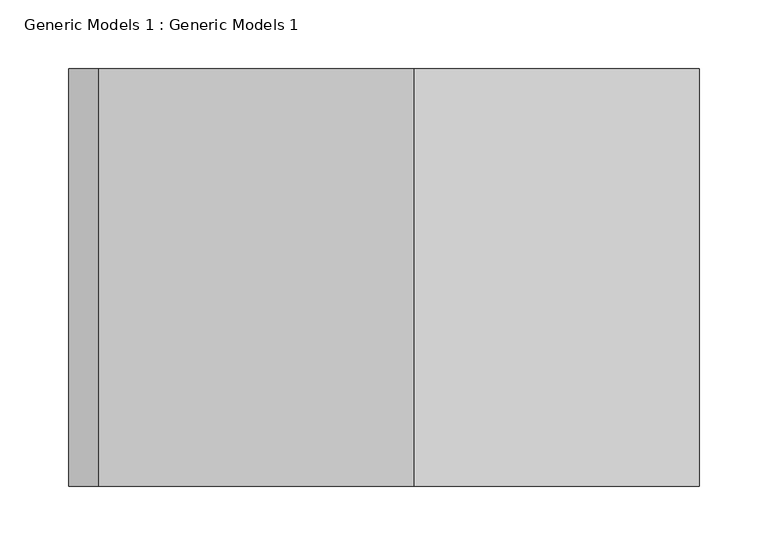
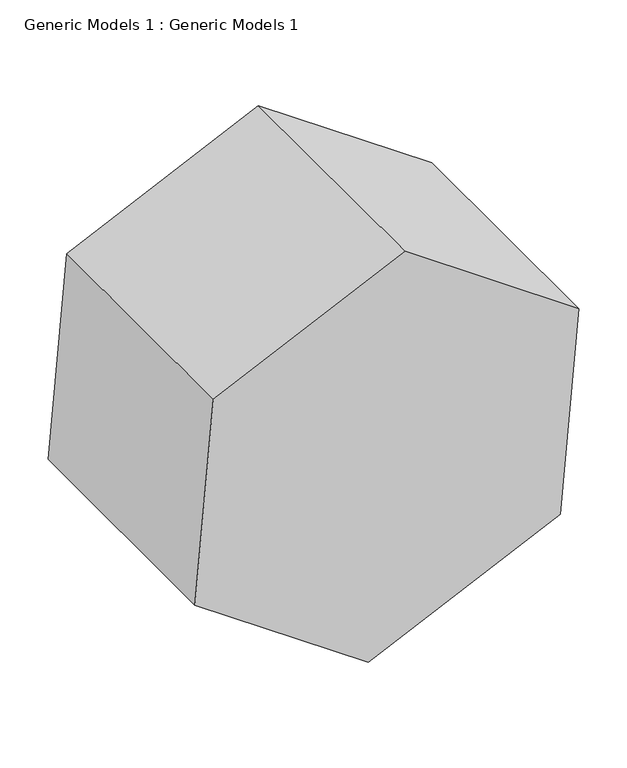
"""IFC4 building model written with IfcOpenShell, lengths in millimetres: proxy geometry, Generic Models 1 : Generic Models 1."""

from ifc_helpers import new_model, si_unit, frame, origin, place, context, project, spatial, polyline, outline, extrude, source, transform, mapped, element, save


def generic_models_1_generic_models_1_1536aad0(model_context):
    return source(origin(), model_context, "Body", "SweptSolid", [
        extrude(outline(polyline([(833.1013393, -6658.3079055), (978.7897542, -6866.3725247), (871.4447157, -7096.5747026), (618.4112624, -7118.7122613), (472.7228475, -6910.647642), (580.067886, -6680.4454641), (833.1013393, -6658.3079055)])), frame((0.0, -10720.3372434, 0.0), z_axis=(0.0, 1.0, 0.0), x_axis=(0.0, 0.0, 1.0)), (0.0, 0.0, 1.0), 304.8),
    ])


if __name__ == "__main__":
    model = new_model("IFC4")
    model_context = context("Model", 3, world=origin())
    ifc_project = project(units=[si_unit("LENGTHUNIT", "METRE", prefix="MILLI")], contexts=[model_context])
    site = spatial("IfcSite", under=ifc_project)
    building = spatial("IfcBuilding", under=site)
    placement = place(None, origin())
    generic_models_1_generic_models_1_shape = generic_models_1_generic_models_1_1536aad0(model_context)
    element("IfcBuildingElementProxy", 1, Name="Generic Models 1 : Generic Models 1", ObjectType="Generic Models 1 : Generic Models 1", at=placement, inside=building, context=model_context, shape_type="MappedRepresentation", body=[
        mapped(generic_models_1_generic_models_1_shape, transform((0.0, 0.0, 0.0), x_axis=(1.0, 0.0, 0.0), y_axis=(0.0, 1.0, 0.0), z_axis=(0.0, 0.0, 1.0))),
    ])
    save(model, "model.ifc")

# Revit data of these elements
# Element 1 (IfcBuildingElementProxy, "Generic Models 1 : Generic Models 1")
#   Materials on its faces: "Render Material 41-165-0"
# Materials
#   "Render Material 41-165-0": colour RGB 41 165 0, transparency 0
